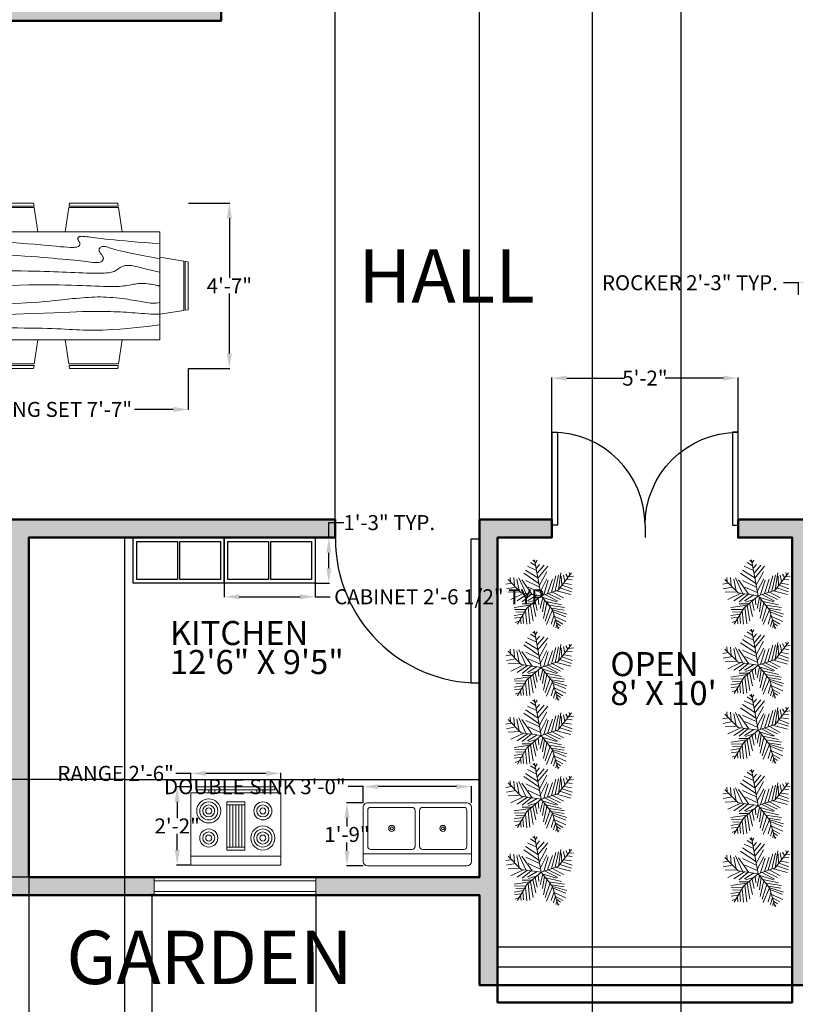
# Model space of a CAD drawing. Units: inches. Extents: x -60 to 743, y -483 to 510.
# Tile 3 of 7: x 120 to 378, y -299 to 29. Entities that reach past the tile are written whole.
import ezdxf

# ---------------------------------------------------------------- set-up
doc = ezdxf.new("R2010")
doc.units = ezdxf.units.IN
doc.header["$MEASUREMENT"] = 0
for name, color, linetype, lineweight in [('A-ANNO-DIMS', 2, 'Continuous', 18), ('A-AREA-IDEN', 7, 'Continuous', 25), ('A-DOOR', 150, 'Continuous', 25), ('A-EQPM', 40, 'Continuous', 18), ('A-FLOR-CASE', 40, 'Continuous', 25), ('A-FLOR-FIXT', 40, 'Continuous', 18), ('A-WALL-PATT', 30, 'Continuous', 13), ('FURNITURE', 40, 'Continuous', 18), ('STAIRS', 202, 'Continuous', 25), ('TREES', 80, 'Continuous', 13), ('WALL BOUNDRY', 10, 'Continuous', 50), ('WINDOW', 200, 'Continuous', 18)]:
    doc.layers.add(name, color=color, linetype=linetype, lineweight=lineweight)
doc.styles.get("Standard").update_dxf_attribs({"font": 'arial.ttf'})
doc.dimstyles.get("Standard").update_dxf_attribs({"dimtxt": 5, "dimasz": 5, "dimexe": 0.18, "dimexo": 0.0625, "dimgap": 0.09, "dimtad": 0, "dimtih": 1, "dimtoh": 1, "dimdec": 1, "dimzin": 0, "dimdsep": 46, "dimlunit": 4, "dimtxsty": 'Standard', "dimcen": 0.09, "dimadec": 0, "dimazin": 0, "dimtfac": 1, "dimtdec": 1, "dimtofl": 0, "dimtmove": 0, "dimatfit": 3, "dimfxl": 1, "dimtolj": 1, "dimtzin": 0, "dimarcsym": 0})

# ---------------------------------------------------------------- blocks, each defined once
blk = doc.blocks.new('Wall Cabinet - 18 x 36 in front')
for p, q in [((17.5, -1.5), (17.5, -16.5)), ((18.5, -16.5), (18.5, -1.5))]:
    blk.add_line(p, q)
blk.add_lwpolyline([(0, -18), (0, 0), (36, 0), (36, -18)], close=True)
for points in [[(17.5, -16.5), (1.5, -16.5), (1.5, -1.5), (17.5, -1.5)], [(18.5, -1.5), (34.5, -1.5), (34.5, -16.5), (18.5, -16.5)]]:
    blk.add_lwpolyline(points)
blk = doc.blocks.new('Range-Oven - 30 in top')
for p, q in [((0, -3), (30, -3)), ((12, -6), (18, -6)), ((13, -20), (13, -6)), ((14, -6), (14, -20)), ((15, -20), (15, -6)), ((16, -6), (16, -20)), ((17, -20), (17, -6)), ((18, -20), (12, -20)), ((6, -24), (6, -25)), ((8, -25), (8, -24)), ((22, -25), (22, -24)), ((24, -24), (24, -25))]:
    blk.add_line(p, q)
for points in [[(0, -24), (0, 0), (30, 0), (30, -24)], [(12, -21), (12, -5), (18, -5), (18, -21)], [(2, -26), (2, -25), (28, -25), (28, -26)]]:
    blk.add_lwpolyline(points, close=True)
for centre, radius in [((6, -9), 4), ((6, -9), 3), ((24, -9), 3), ((6, -9), 2), ((6, -9), 1), ((24, -9), 2), ((24, -9), 1), ((6, -18), 3), ((6, -18), 2), ((24, -18), 4), ((24, -18), 3), ((24, -18), 2), ((6, -18), 1), ((24, -18), 1)]:
    blk.add_circle(centre, radius)
blk = doc.blocks.new('Sink-double - 36 in top')
for p, q in [((-18, -4), (18, -4)), ((-0.75, -18.5), (-0.75, -6.5)), ((0.75, -6.5), (0.75, -18.5))]:
    blk.add_line(p, q)
for points in [[(-16.5, 0), (16.5, 0)], [(-18, -19.5), (-18, -1.5)], [(18, -1.5), (18, -19.5)], [(-16.5, -18.5), (-16.5, -6.5)], [(-15.5, -5.5), (-1.75, -5.5)], [(1.75, -5.5), (15.5, -5.5)], [(16.5, -6.5), (16.5, -18.5)], [(-1.75, -19.5), (-15.5, -19.5)], [(15.5, -19.5), (1.75, -19.5)], [(16.5, -21), (-16.5, -21)]]:
    blk.add_lwpolyline(points)
for centre, radius in [((-8.5, -12.5), 1), ((-8.5, -12.5), 0.5), ((8.5, -12.5), 1), ((8.5, -12.5), 0.5)]:
    blk.add_circle(centre, radius)
for centre, radius, start, end in [((-16.5, -1.5), 1.5, 90, 180), ((16.5, -1.5), 1.5, 0, 90), ((-15.5, -6.5), 1, 90, 180), ((-1.75, -6.5), 1, 0, 90), ((1.75, -6.5), 1, 90, 180), ((15.5, -6.5), 1, 0, 90), ((-16.5, -19.5), 1.5, 180, 270), ((-15.5, -18.5), 1, 180, 270), ((-1.75, -18.5), 1, 270, 0), ((1.75, -18.5), 1, 180, 270), ((15.5, -18.5), 1, 270, 0), ((16.5, -19.5), 1.5, 270, 0)]:
    blk.add_arc(centre, radius, start, end)
blk = doc.blocks.new('*U5')
for p, q in [((0, 0), (0, -100)), ((750, 0), (750, -100))]:
    blk.add_line(p, q)
blk.add_lwpolyline([(0, 0), (0, 750), (43.75, 750), (43.75, 0)], close=True)
blk.add_arc((0, 0), 750, 0, 90)
blk = doc.blocks.new('Dining Set - 36 x 72 in.')
for p, q in [((-22, 27.5), (-22.1562, 26.50042)), ((-5.8416, 26.5), (-22.1534, 26.5)), ((-22, 27.5), (-6, 27.5)), ((-5.8437, 26.49966), (-6, 27.5)), ((6, 27.5), (5.8438, 26.50042)), ((22.1584, 26.5), (5.8466, 26.5)), ((6, 27.5), (22, 27.5)), ((22.1563, 26.49966), (22, 27.5)), ((-22.2343, 26.00059), (-23.4847, 17.99762)), ((-22.2304, 26), (-5.7608, 26)), ((-4.5152, 17.99762), (-5.7655, 25.99926)), ((5.7657, 26.00059), (4.5153, 17.99762)), ((5.7696, 26), (22.2392, 26)), ((23.4848, 17.99762), (22.2345, 25.99926)), ((36, 18), (-36, 18)), ((-36, 18), (-36, -18)), ((36, -18), (36, 18)), ((-45.5, 8), (-44.5004, 8.15617)), ((-45.5, 8), (-45.5, -8)), ((-44.5, -8.15843), (-44.5, 8.15338)), ((-44.0006, 8.23428), (-35.9976, 9.48474)), ((-44, 8.23041), (-44, -8.23915)), ((44.0006, 8.23428), (35.9976, 9.48474)), ((44, 8.23041), (44, -8.23915)), ((44.5, -8.15843), (44.5, 8.15338)), ((45.5, 8), (44.5005, 8.15617)), ((45.5, 8), (45.5, -8)), ((-44.4997, -8.15631), (-45.5, -8)), ((-35.9976, -9.48476), (-43.9993, -8.2345)), ((35.9976, -9.48476), (43.9993, -8.2345)), ((44.4997, -8.15631), (45.5, -8)), ((-36, -18), (36, -18)), ((-22.2343, -26.0006), (-23.4847, -17.99762)), ((-4.5152, -17.99762), (-5.7655, -25.99928)), ((5.7657, -26.0006), (4.5153, -17.99762)), ((23.4848, -17.99762), (22.2345, -25.99928)), ((-22.2304, -26), (-5.7608, -26)), ((5.7696, -26), (22.2392, -26)), ((-22, -27.5), (-22.1562, -26.50044)), ((-5.8416, -26.5), (-22.1534, -26.5)), ((-22, -27.5), (-6, -27.5)), ((-5.8437, -26.49967), (-6, -27.5)), ((6, -27.5), (5.8438, -26.50044)), ((22.1584, -26.5), (5.8466, -26.5)), ((6, -27.5), (22, -27.5)), ((22.1563, -26.49967), (22, -27.5))]:
    blk.add_line(p, q)
for points in [[(-36, 15), (-31.1772, 14.97754), (-26.8079, 14.91406), (-22.8538, 14.81543), (-19.276, 14.6875), (-16.0362, 14.53613), (-13.0957, 14.36718), (-10.4159, 14.18652), (-7.9583, 14), (-5.6904, 13.81315), (-3.6035, 13.63021), (-1.6954, 13.45508), (0.0365, 13.29166), (1.5945, 13.14388), (2.9811, 13.01562), (4.1988, 12.9108), (5.25, 12.83333), (6.1393, 12.78613), (6.8802, 12.76823), (7.4883, 12.77767), (7.9792, 12.8125), (8.3685, 12.87077), (8.6719, 12.95052), (8.9049, 13.0498), (9.0833, 13.16666), (9.2205, 13.29899), (9.3216, 13.44401), (9.3895, 13.59879), (9.4271, 13.76041), (9.4373, 13.92594), (9.4232, 14.09245), (9.3875, 14.257), (9.3333, 14.41666), (9.2638, 14.56917), (9.1836, 14.71484), (9.0975, 14.85465), (9.0104, 14.98958), (8.9272, 15.1206), (8.8529, 15.2487), (8.7922, 15.37483), (8.75, 15.5), (8.7305, 15.62467), (8.7344, 15.74739), (8.7617, 15.86621), (8.8125, 15.97916), (8.8867, 16.08431), (8.9844, 16.17968), (9.1055, 16.26334), (9.25, 16.33333), (9.4189, 16.38802), (9.6172, 16.42708), (9.8506, 16.45052), (10.125, 16.45833), (10.4463, 16.45052), (10.8203, 16.42708), (11.2529, 16.38802), (11.75, 16.33333), (12.3184, 16.26318), (12.9694, 16.17838), (13.7151, 16.07991), (14.5677, 15.96875), (15.5395, 15.84586), (16.6426, 15.71224), (17.8893, 15.56884), (19.2917, 15.41666), (20.859, 15.25667), (22.5879, 15.08984), (24.4721, 14.91715), (26.5052, 14.73958), (28.6809, 14.5581), (30.9929, 14.3737), (33.4347, 14.18733), (36, 14)], [(-36, 10), (-28.9766, 10.14274), (-23.1725, 10.20442), (-18.4241, 10.19775), (-14.5677, 10.13541), (-11.4399, 10.03011), (-8.877, 9.89453), (-6.7154, 9.74137), (-4.7917, 9.58333), (-2.9698, 9.43082), (-1.2246, 9.28515), (0.4415, 9.14534), (2.026, 9.01041), (3.5266, 8.87939), (4.9408, 8.7513), (6.266, 8.62516), (7.5, 8.5), (8.6411, 8.37549), (9.6914, 8.2539), (10.6538, 8.13818), (11.5312, 8.03125), (12.3267, 7.93603), (13.043, 7.85547), (13.6831, 7.79248), (14.25, 7.75), (14.7471, 7.7303), (15.1797, 7.73307), (15.5537, 7.75732), (15.875, 7.80208), (16.1494, 7.86637), (16.3828, 7.94922), (16.5811, 8.04964), (16.75, 8.16666), (16.8944, 8.29915), (17.0143, 8.44531), (17.1089, 8.60319), (17.1771, 8.77083), (17.218, 8.94629), (17.2305, 9.1276), (17.2137, 9.31282), (17.1667, 9.5), (17.0895, 9.6875), (16.987, 9.875), (16.8649, 10.0625), (16.7292, 10.25), (16.5856, 10.4375), (16.4401, 10.625), (16.2985, 10.8125), (16.1667, 11), (16.05, 11.18733), (15.9518, 11.3737), (15.8752, 11.5581), (15.8229, 11.73958), (15.798, 11.91715), (15.8034, 12.08984), (15.842, 12.25667), (15.9167, 12.41666), (16.0295, 12.56836), (16.1784, 12.70833), (16.3605, 12.83268), (16.5729, 12.9375), (16.8127, 13.01888), (17.0768, 13.07291), (17.3625, 13.0957), (17.6667, 13.08333), (17.9894, 13.03312), (18.3418, 12.94726), (18.7382, 12.82918), (19.1927, 12.68229), (19.7195, 12.51001), (20.3327, 12.31575), (21.0465, 12.10294), (21.875, 11.875), (22.8357, 11.63354), (23.959, 11.37304), (25.2786, 11.08618), (26.8282, 10.76562), (28.6414, 10.40405), (30.752, 9.99414), (33.1936, 9.52856), (36, 9)], [(-36, 5.5), (-30.7157, 5.3348), (-26.069, 5.20963), (-21.9946, 5.11767), (-18.4271, 5.05208), (-15.3009, 5.00602), (-12.5508, 4.97265), (-10.1112, 4.94515), (-7.9167, 4.91666), (-5.909, 4.88167), (-4.0586, 4.83984), (-2.3429, 4.79215), (-0.7396, 4.73958), (0.7739, 4.6831), (2.22, 4.6237), (3.6213, 4.56233), (5, 4.5), (6.373, 4.43782), (7.7344, 4.3776), (9.0723, 4.32129), (10.375, 4.27083), (11.6309, 4.22819), (12.8281, 4.19531), (13.9551, 4.17415), (15, 4.16666), (15.954, 4.17448), (16.819, 4.19791), (17.6001, 4.23698), (18.3021, 4.29166), (18.9299, 4.36198), (19.4883, 4.44791), (19.9823, 4.54948), (20.4167, 4.66666), (20.7969, 4.79899), (21.1302, 4.94401), (21.4245, 5.09879), (21.6875, 5.26041), (21.9271, 5.42594), (22.1511, 5.59245), (22.3672, 5.757), (22.5834, 5.91666), (22.8065, 6.06868), (23.0404, 6.21093), (23.2879, 6.34147), (23.5521, 6.45833), (23.8358, 6.55957), (24.142, 6.64323), (24.4735, 6.70735), (24.8334, 6.75), (25.2235, 6.76969), (25.642, 6.76692), (26.0858, 6.74267), (26.5521, 6.69791), (27.0379, 6.63362), (27.5404, 6.55078), (28.0565, 6.45036), (28.5834, 6.33333), (29.1242, 6.19987), (29.7071, 6.04687), (30.3661, 5.87044), (31.1354, 5.66666), (32.0493, 5.43164), (33.142, 5.16146), (34.4475, 4.85221), (36, 4.5)], [(-36, -1), (-30.7915, -0.6591), (-26.0195, -0.38216), (-21.6519, -0.16284), (-17.6563, 0.00521), (-14.0005, 0.12833), (-10.6523, 0.21289), (-7.5796, 0.26522), (-4.75, 0.29166), (-2.134, 0.29793), (0.2878, 0.28711), (2.5317, 0.26163), (4.6146, 0.22396), (6.5529, 0.17651), (8.3633, 0.12174), (10.0623, 0.06209), (11.6667, 0), (13.1899, -0.06201), (14.6341, -0.1211), (15.9982, -0.17432), (17.2813, -0.21875), (18.4823, -0.25147), (19.6003, -0.26953), (20.6343, -0.27002), (21.5834, -0.25), (22.4481, -0.20768), (23.2357, -0.14584), (23.9549, -0.06836), (24.6146, 0.02083), (25.2235, 0.11784), (25.7904, 0.21875), (26.3241, 0.31966), (26.8334, 0.41666), (27.3265, 0.50618), (27.8099, 0.58593), (28.2894, 0.65397), (28.7709, 0.70833), (29.2601, 0.74707), (29.763, 0.76823), (30.2855, 0.76985), (30.8334, 0.75), (31.4088, 0.70784), (31.9994, 0.64713), (32.589, 0.57275), (33.1615, 0.48958), (33.7008, 0.4025), (34.1908, 0.3164), (34.6153, 0.23616), (34.9584, 0.16666), (35.2099, 0.11165), (35.3848, 0.07031), (35.504, 0.04069), (35.5886, 0.02083), (35.6594, 0.00879), (35.7377, 0.0026), (35.8442, 0.00032), (36, 0)], [(-36, -6.5), (-27.1843, -6.31267), (-20.084, -6.1263), (-14.469, -5.9419), (-10.1094, -5.76042), (-6.7752, -5.58285), (-4.2363, -5.41016), (-2.2629, -5.24333), (-0.625, -5.08334), (0.8708, -4.93099), (2.2715, -4.78646), (3.5872, -4.64974), (4.8281, -4.52084), (6.0046, -4.39974), (7.127, -4.28646), (8.2053, -4.18099), (9.25, -4.08334), (10.2705, -3.99382), (11.2734, -3.91407), (12.2647, -3.84603), (13.25, -3.79167), (14.2354, -3.75293), (15.2266, -3.73177), (16.2295, -3.73015), (17.25, -3.75), (18.2912, -3.79248), (19.3451, -3.85547), (20.4009, -3.93604), (21.4479, -4.03125), (22.4754, -4.13819), (23.4727, -4.25391), (24.4289, -4.37549), (25.3334, -4.5), (26.1785, -4.62492), (26.9694, -4.74935), (27.7145, -4.87281), (28.4219, -4.99479), (29.1, -5.11483), (29.7572, -5.23242), (30.4016, -5.34709), (31.0417, -5.45834), (31.6837, -5.56437), (32.3262, -5.65821), (32.9658, -5.73153), (33.599, -5.77604), (34.2224, -5.78345), (34.8327, -5.74545), (35.4264, -5.65373), (36, -5.5)], [(-36, -10), (-26.4022, -9.81299), (-18.4675, -9.62891), (-11.9839, -9.45069), (-6.7396, -9.28125), (-2.5226, -9.12354), (0.8789, -8.98047), (3.6769, -8.85498), (6.0833, -8.75), (8.2767, -8.66765), (10.3021, -8.60677), (12.1712, -8.56543), (13.8958, -8.54167), (15.4876, -8.53353), (16.9583, -8.53907), (18.3197, -8.55632), (19.5834, -8.58334), (20.7616, -8.61841), (21.8685, -8.66081), (22.9188, -8.71004), (23.9271, -8.76563), (24.9081, -8.82707), (25.8763, -8.89388), (26.8465, -8.96558), (27.8334, -9.04167), (28.8474, -9.12118), (29.8828, -9.20117), (30.93, -9.27824), (31.9792, -9.34896), (33.0205, -9.40991), (34.0443, -9.45768), (35.0407, -9.48885), (36, -9.5)], [(-36, -14.5), (-30.0881, -14.33513), (-25.0332, -14.21224), (-20.7312, -14.12647), (-17.0781, -14.07292), (-13.97, -14.04671), (-11.3027, -14.04297), (-8.9724, -14.05681), (-6.875, -14.08334), (-4.9224, -14.11833), (-3.0905, -14.16016), (-1.3709, -14.20785), (0.2448, -14.26042), (1.7647, -14.3169), (3.1973, -14.3763), (4.5507, -14.43767), (5.8333, -14.5), (7.0554, -14.5621), (8.235, -14.62175), (9.3922, -14.67652), (10.5469, -14.72396), (11.7192, -14.76164), (12.929, -14.78711), (14.1965, -14.79794), (15.5417, -14.79167), (16.9933, -14.76424), (18.6152, -14.70508), (20.4804, -14.60197), (22.6615, -14.44271), (25.2312, -14.21509), (28.2624, -13.9069), (31.8277, -13.50594), (36, -13)]]:
    blk.add_lwpolyline(points)
blk = doc.blocks.new('*U21')
for p, q in [((-221.9198, 1197.3052), (-433.5526, 1338.8594)), ((-258.7244, 1362.456), (-332.3336, 1421.4348)), ((0, 0), (-266.7, 1447.8)), ((-231.1146, 1315.2628), (-166.7002, 1421.4348)), ((-194.31, 1102.9442), (-65.4812, 1256.284)), ((-148.3106, 914.1968), (118.5418, 1220.9018)), ((-93.091, 489.5342), (-700.3796, 902.3858)), ((-129.8956, 713.6638), (-626.7704, 1032.1544)), ((-185.1152, 1008.5578), (-553.1612, 1185.4942)), ((-129.8956, 701.8528), (265.7602, 1185.4942)), ((-74.7014, 418.7444), (219.7608, 961.39)), ((412.9786, 147.447), (587.8068, 796.2392)), ((560.197, 182.8292), (698.2206, 819.8358)), ((685.8, 228.6), (1219.2, 914.4)), ((689.0258, 230.0224), (790.2448, 914.1968)), ((891.4384, 831.6214), (946.658, 572.1096)), ((983.4626, 867.0036), (1066.2666, 725.4494)), ((1121.4862, 925.9824), (1149.0706, 831.6214)), ((-1206.4492, 501.3198), (-1418.082, 465.9376)), ((-800.1, 114.3), (-1333.5, 647.7)), ((-1234.059, 536.7274), (-1252.4486, 737.2604)), ((-1105.2302, 725.4494), (-1077.6458, 395.1732)), ((-976.4268, 666.4706), (-884.4026, 194.6402)), ((-902.8176, 713.6638), (-617.5756, 100.2538)), ((-369.1382, 53.086), (-783.1836, 642.874)), ((-617.5756, 607.4918), (-74.7014, 347.98)), ((-28.6766, 171.0436), (228.9556, 678.2816)), ((100.1268, 41.275), (284.1498, 619.2774)), ((256.5654, 88.4682), (449.7832, 666.4706)), ((808.6344, 784.4282), (827.0494, 418.7444)), ((845.439, 418.7444), (1241.0948, 277.1902)), ((919.0482, 501.3198), (1222.6798, 454.152)), ((1029.462, 654.685), (1241.0948, 631.0884)), ((1112.2914, 760.8316), (1296.3144, 784.4282)), ((-1031.621, 347.98), (-1399.667, 277.1902)), ((-847.598, 159.2326), (-1326.0578, 135.636)), ((-718.7946, 88.4682), (-1215.644, -147.447)), ((-543.9664, 76.6572), (-967.2066, -206.4512)), ((0, 0), (-800.1, 114.3)), ((-405.9428, 53.086), (-764.794, -241.8334)), ((0, 0), (-571.5, -495.3)), ((-166.7002, 29.4894), (-543.9664, -206.4512)), ((-525.5514, 347.98), (-28.6766, 123.8504)), ((0, 0), (685.8, 228.6)), ((0, 0), (457.2, -571.5)), ((164.5412, 41.275), (661.416, -218.2368)), ((284.1498, 88.4682), (781.0246, -147.447)), ((458.978, 147.447), (891.4384, -88.4682)), ((615.4166, 194.6402), (1185.8752, 41.275)), ((753.4148, 312.5978), (1222.6798, 159.2326)), ((-442.7474, -383.3876), (-1086.8406, -477.7486)), ((-387.5278, -324.4088), (-764.794, -324.4088)), ((-166.7002, -147.447), (-507.1618, -253.619)), ((-433.5526, -383.3876), (-323.1134, -1020.3688)), ((-341.5284, -289.0012), (-221.9198, -831.6214)), ((-240.3094, -218.2368), (-157.5054, -595.7062)), ((-120.7008, -88.4682), (-93.091, -371.5766)), ((63.3222, -76.6826), (-37.8714, -513.1308)), ((44.9326, -64.897), (615.4166, -241.8334)), ((127.7366, -159.258), (54.1274, -654.685)), ((228.9556, -289.0012), (90.932, -914.1968)), ((192.151, -230.0224), (817.8292, -371.5766)), ((311.7596, -383.3876), (937.4378, -477.7486)), ((-718.7946, -737.2604), (-1086.8406, -796.2392)), ((-617.5756, -548.5384), (-1077.6458, -560.324)), ((-681.9646, -666.496), (-1022.4262, -654.685)), ((-571.5, -495.3), (-952.5, -1143)), ((-737.1842, -784.4536), (-709.5744, -1114.7298)), ((-635.9652, -607.5172), (-580.771, -1150.1374)), ((-525.5514, -465.963), (-451.9422, -1126.5408)), ((357.759, -430.5554), (164.5412, -1020.3688)), ((458.978, -572.1096), (210.5406, -1161.923)), ((514.1976, -772.6426), (403.7838, -1138.3264)), ((412.9786, -501.3452), (919.0482, -583.9206)), ((457.2, -571.5), (685.8, -1333.5)), ((468.1982, -572.1096), (1029.462, -737.2604)), ((486.5878, -642.8994), (983.4626, -843.4324)), ((-783.1836, -867.029), (-1077.6458, -902.4112)), ((-875.2078, -1008.5832), (-1040.8412, -1079.3476)), ((-829.2084, -937.7934), (-810.7934, -1126.5408)), ((578.612, -961.39), (495.7826, -1232.7128)), ((541.8074, -831.6214), (992.6574, -1032.1544)), ((578.612, -973.1756), (873.0488, -1138.3264)), ((624.6114, -1161.923), (587.8068, -1291.6916)), ((624.6114, -1102.9442), (781.0246, -1209.1162)), ((679.8056, -1268.095), (716.6102, -1291.6916))]:
    blk.add_line(p, q)
blk = doc.blocks.new('*D26')
at = {"layer": 'A-ANNO-DIMS', "color": 0, "lineweight": -2, "transparency": 16777216}
for p, q in [((188.17, -158.78), (188.17, -163.44)), ((218.45, -158.78), (218.45, -163.44)), ((193.17, -163.26), (213.45, -163.26)), ((218.45, -163.26), (223.45, -163.26))]:
    blk.add_line(p, q, dxfattribs=at)
at = {"layer": 'A-ANNO-DIMS', "color": 0, "transparency": 16777216}
for points in [[(193.17, -162.43), (193.17, -164.09), (188.17, -163.26)], [(213.45, -162.43), (213.45, -164.09), (218.45, -163.26)]]:
    blk.add_solid(points, dxfattribs=at)
at = {"layer": 'Defpoints', "color": 0, "transparency": 16777216}
for p in [(188.17, -158.72), (218.45, -158.72), (218.45, -163.26)]:
    blk.add_point(p, dxfattribs=at)
at = {"layer": 'A-ANNO-DIMS', "color": 0, "transparency": 16777216, "insert": (260.68, -163.26), "char_height": 5, "attachment_point": 5}
blk.add_mtext('\\A1;CABINET 2\'-6 1/2" TYP.', dxfattribs=at)
blk = doc.blocks.new('*D27')
at = {"layer": 'A-ANNO-DIMS', "color": 0, "lineweight": -2, "transparency": 16777216}
for p, q in [((222.99, -143.58), (222.99, -138.58)), ((222.99, -138.58), (227.99, -138.58)), ((218.51, -143.58), (223.17, -143.58)), ((222.99, -153.72), (222.99, -148.58)), ((218.51, -158.72), (223.17, -158.72))]:
    blk.add_line(p, q, dxfattribs=at)
at = {"layer": 'A-ANNO-DIMS', "color": 0, "transparency": 16777216}
for points in [[(222.16, -148.58), (223.83, -148.58), (222.99, -143.58)], [(222.16, -153.72), (223.83, -153.72), (222.99, -158.72)]]:
    blk.add_solid(points, dxfattribs=at)
at = {"layer": 'Defpoints', "color": 0, "transparency": 16777216}
for p in [(218.45, -143.58), (222.99, -143.58), (218.45, -158.72)]:
    blk.add_point(p, dxfattribs=at)
at = {"layer": 'A-ANNO-DIMS', "color": 0, "transparency": 16777216, "insert": (243.09, -138.58), "char_height": 5, "attachment_point": 5}
blk.add_mtext('\\A1;1\'-3" TYP.', dxfattribs=at)
blk = doc.blocks.new('*D34')
at = {"layer": 'A-ANNO-DIMS', "color": 0, "lineweight": -2, "transparency": 16777216}
for p, q in [((379.23, -58.74), (374.23, -58.74)), ((379.23, -62.73), (379.23, -58.56)), ((401.23, -58.74), (384.23, -58.74)), ((406.23, -62.73), (406.23, -58.56))]:
    blk.add_line(p, q, dxfattribs=at)
at = {"layer": 'A-ANNO-DIMS', "color": 0, "transparency": 16777216}
for points in [[(384.23, -57.91), (384.23, -59.58), (379.23, -58.74)], [(401.23, -57.91), (401.23, -59.58), (406.23, -58.74)]]:
    blk.add_solid(points, dxfattribs=at)
at = {"layer": 'Defpoints', "color": 0, "transparency": 16777216}
for p in [(379.23, -58.74), (379.23, -62.79), (406.23, -62.79)]:
    blk.add_point(p, dxfattribs=at)
at = {"layer": 'A-ANNO-DIMS', "color": 0, "transparency": 16777216, "insert": (343.12, -58.74), "char_height": 5, "attachment_point": 5}
blk.add_mtext('\\A1;ROCKER 2\'-3" TYP.', dxfattribs=at)
blk = doc.blocks.new('*D58')
at = {"layer": 'A-ANNO-DIMS', "color": 0, "lineweight": -2, "transparency": 16777216}
for p, q in [((177.04, -222.05), (172.04, -222.05)), ((177.04, -226.49), (177.04, -221.87)), ((202.04, -222.05), (182.04, -222.05)), ((207.04, -226.49), (207.04, -221.87))]:
    blk.add_line(p, q, dxfattribs=at)
at = {"layer": 'A-ANNO-DIMS', "color": 0, "transparency": 16777216}
for points in [[(182.04, -221.22), (182.04, -222.88), (177.04, -222.05)], [(202.04, -221.22), (202.04, -222.88), (207.04, -222.05)]]:
    blk.add_solid(points, dxfattribs=at)
at = {"layer": 'Defpoints', "color": 0, "transparency": 16777216}
for p in [(177.04, -222.05), (177.04, -226.55), (207.04, -226.55)]:
    blk.add_point(p, dxfattribs=at)
at = {"layer": 'A-ANNO-DIMS', "color": 0, "transparency": 16777216, "insert": (152.05, -222.05), "char_height": 5, "attachment_point": 5}
blk.add_mtext('\\A1;RANGE 2\'-6"', dxfattribs=at)
blk = doc.blocks.new('*D59')
at = {"layer": 'A-ANNO-DIMS', "color": 0, "lineweight": -2, "transparency": 16777216}
for p, q in [((176.98, -226.55), (172.36, -226.55)), ((172.54, -231.55), (172.54, -236.95)), ((172.54, -247.55), (172.54, -242.15)), ((176.98, -252.55), (172.36, -252.55))]:
    blk.add_line(p, q, dxfattribs=at)
at = {"layer": 'A-ANNO-DIMS', "color": 0, "transparency": 16777216}
for points in [[(171.71, -231.55), (173.38, -231.55), (172.54, -226.55)], [(171.71, -247.55), (173.38, -247.55), (172.54, -252.55)]]:
    blk.add_solid(points, dxfattribs=at)
at = {"layer": 'Defpoints', "color": 0, "transparency": 16777216}
for p in [(177.04, -226.55), (172.54, -252.55), (177.04, -252.55)]:
    blk.add_point(p, dxfattribs=at)
at = {"layer": 'A-ANNO-DIMS', "color": 0, "transparency": 16777216, "insert": (172.54, -239.55), "char_height": 5, "attachment_point": 5}
blk.add_mtext('\\A1;2\'-2"', dxfattribs=at)
blk = doc.blocks.new('*D60')
at = {"layer": 'A-ANNO-DIMS', "color": 0, "lineweight": -2, "transparency": 16777216}
for p, q in [((234.43, -226.46), (229.43, -226.46)), ((234.43, -231.8), (234.43, -226.28)), ((265.43, -226.46), (239.43, -226.46)), ((270.43, -231.8), (270.43, -226.28))]:
    blk.add_line(p, q, dxfattribs=at)
at = {"layer": 'A-ANNO-DIMS', "color": 0, "transparency": 16777216}
for points in [[(239.43, -225.63), (239.43, -227.29), (234.43, -226.46)], [(265.43, -225.63), (265.43, -227.29), (270.43, -226.46)]]:
    blk.add_solid(points, dxfattribs=at)
at = {"layer": 'Defpoints', "color": 0, "transparency": 16777216}
for p in [(234.43, -226.46), (234.43, -231.86), (270.43, -231.86)]:
    blk.add_point(p, dxfattribs=at)
at = {"layer": 'A-ANNO-DIMS', "color": 0, "transparency": 16777216, "insert": (198.37, -226.46), "char_height": 5, "attachment_point": 5}
blk.add_mtext('\\A1;DOUBLE SINK 3\'-0"', dxfattribs=at)
blk = doc.blocks.new('*D61')
at = {"layer": 'A-ANNO-DIMS', "color": 0, "lineweight": -2, "transparency": 16777216}
for p, q in [((234.37, -231.86), (228.85, -231.86)), ((229.03, -236.86), (229.03, -239.72)), ((229.03, -247.86), (229.03, -245)), ((234.37, -252.86), (228.85, -252.86))]:
    blk.add_line(p, q, dxfattribs=at)
at = {"layer": 'A-ANNO-DIMS', "color": 0, "transparency": 16777216}
for points in [[(228.2, -236.86), (229.87, -236.86), (229.03, -231.86)], [(228.2, -247.86), (229.87, -247.86), (229.03, -252.86)]]:
    blk.add_solid(points, dxfattribs=at)
at = {"layer": 'Defpoints', "color": 0, "transparency": 16777216}
for p in [(234.43, -231.86), (229.03, -252.86), (234.43, -252.86)]:
    blk.add_point(p, dxfattribs=at)
at = {"layer": 'A-ANNO-DIMS', "color": 0, "transparency": 16777216, "insert": (229.03, -242.36), "char_height": 5, "attachment_point": 5}
blk.add_mtext('\\A1;1\'-9"', dxfattribs=at)
blk = doc.blocks.new('*D62')
at = {"layer": 'A-ANNO-DIMS', "color": 0, "lineweight": -2, "transparency": 16777216}
for p, q in [((85.25, -87.32), (85.25, -101.08)), ((176.25, -87.32), (176.25, -101.08)), ((90.25, -100.9), (103.18, -100.9)), ((171.25, -100.9), (158.32, -100.9))]:
    blk.add_line(p, q, dxfattribs=at)
at = {"layer": 'A-ANNO-DIMS', "color": 0, "transparency": 16777216}
for points in [[(90.25, -100.07), (90.25, -101.74), (85.25, -100.9)], [(171.25, -100.07), (171.25, -101.74), (176.25, -100.9)]]:
    blk.add_solid(points, dxfattribs=at)
at = {"layer": 'Defpoints', "color": 0, "transparency": 16777216}
for p in [(85.25, -87.25), (176.25, -87.25), (176.25, -100.9)]:
    blk.add_point(p, dxfattribs=at)
at = {"layer": 'A-ANNO-DIMS', "color": 0, "transparency": 16777216, "insert": (130.75, -100.9), "char_height": 5, "attachment_point": 5}
blk.add_mtext('\\A1;DINING SET 7\'-7"', dxfattribs=at)
blk = doc.blocks.new('*D63')
at = {"layer": 'A-ANNO-DIMS', "color": 0, "lineweight": -2, "transparency": 16777216}
for p, q in [((176.31, -32.25), (190.08, -32.25)), ((189.9, -37.25), (189.9, -57.16)), ((189.9, -82.25), (189.9, -62.34)), ((176.31, -87.25), (190.08, -87.25))]:
    blk.add_line(p, q, dxfattribs=at)
at = {"layer": 'A-ANNO-DIMS', "color": 0, "transparency": 16777216}
for points in [[(189.07, -37.25), (190.73, -37.25), (189.9, -32.25)], [(189.07, -82.25), (190.73, -82.25), (189.9, -87.25)]]:
    blk.add_solid(points, dxfattribs=at)
at = {"layer": 'Defpoints', "color": 0, "transparency": 16777216}
for p in [(176.25, -32.25), (189.9, -32.25), (176.25, -87.25)]:
    blk.add_point(p, dxfattribs=at)
at = {"layer": 'A-ANNO-DIMS', "color": 0, "transparency": 16777216, "insert": (189.9, -59.75), "char_height": 5, "attachment_point": 5}
blk.add_mtext('\\A1;4\'-7"', dxfattribs=at)
blk = doc.blocks.new('*D69')
at = {"layer": 'A-ANNO-DIMS', "color": 0, "lineweight": -2, "transparency": 16777216}
for p, q in [((310.62, 340.16), (310.62, -473.51)), ((340.15, 340.16), (340.15, -473.51)), ((305.62, -473.33), (300.62, -473.33)), ((345.15, -473.33), (350.15, -473.33))]:
    blk.add_line(p, q, dxfattribs=at)
at = {"layer": 'A-ANNO-DIMS', "color": 0, "transparency": 16777216}
for points in [[(305.62, -472.5), (305.62, -474.17), (310.62, -473.33)], [(345.15, -472.5), (345.15, -474.17), (340.15, -473.33)]]:
    blk.add_solid(points, dxfattribs=at)
at = {"layer": 'Defpoints', "color": 0, "transparency": 16777216}
for p in [(310.62, 340.23), (340.15, 340.23), (340.15, -473.33)]:
    blk.add_point(p, dxfattribs=at)
at = {"layer": 'A-ANNO-DIMS', "color": 0, "transparency": 16777216, "insert": (325.38, -473.33), "char_height": 5, "attachment_point": 5}
blk.add_mtext('\\A1;2\'-5 1/2"', dxfattribs=at)
blk = doc.blocks.new('*D76')
at = {"layer": 'A-ANNO-DIMS', "color": 0, "lineweight": -2, "transparency": 16777216}
for p, q in [((154.99, -224.11), (154.99, -473.51)), ((123.15, -256.64), (123.15, -473.51)), ((128.15, -473.33), (132.29, -473.33)), ((149.99, -473.33), (145.85, -473.33))]:
    blk.add_line(p, q, dxfattribs=at)
at = {"layer": 'A-ANNO-DIMS', "color": 0, "transparency": 16777216}
for points in [[(128.15, -472.5), (128.15, -474.17), (123.15, -473.33)], [(149.99, -472.5), (149.99, -474.17), (154.99, -473.33)]]:
    blk.add_solid(points, dxfattribs=at)
at = {"layer": 'Defpoints', "color": 0, "transparency": 16777216}
for p in [(154.99, -224.05), (123.15, -256.58), (154.99, -473.33)]:
    blk.add_point(p, dxfattribs=at)
at = {"layer": 'A-ANNO-DIMS', "color": 0, "transparency": 16777216, "insert": (139.07, -473.33), "char_height": 5, "attachment_point": 5}
blk.add_mtext('\\A1;2\'-8"', dxfattribs=at)
blk = doc.blocks.new('*D77')
at = {"layer": 'A-ANNO-DIMS', "color": 0, "lineweight": -2, "transparency": 16777216}
for p, q in [((154.93, -224.05), (-36.93, -224.05)), ((-36.75, -229.05), (-36.75, -237.64)), ((-36.75, -251.58), (-36.75, -242.99)), ((123.08, -256.58), (-36.93, -256.58))]:
    blk.add_line(p, q, dxfattribs=at)
at = {"layer": 'A-ANNO-DIMS', "color": 0, "transparency": 16777216}
for points in [[(-37.58, -229.05), (-35.91, -229.05), (-36.75, -224.05)], [(-37.58, -251.58), (-35.91, -251.58), (-36.75, -256.58)]]:
    blk.add_solid(points, dxfattribs=at)
at = {"layer": 'Defpoints', "color": 0, "transparency": 16777216}
for p in [(154.99, -224.05), (-36.75, -256.58), (123.15, -256.58)]:
    blk.add_point(p, dxfattribs=at)
at = {"layer": 'A-ANNO-DIMS', "color": 0, "transparency": 16777216, "insert": (-36.75, -240.31), "char_height": 5, "attachment_point": 5}
blk.add_mtext('\\A1;2\'-8 1/2"', dxfattribs=at)
blk = doc.blocks.new('*D78')
at = {"layer": 'A-ANNO-DIMS', "color": 0, "lineweight": -2, "transparency": 16777216}
for p, q in [((225.15, -143.52), (225.15, 465.7)), ((230.15, 465.52), (242.31, 465.52)), ((268.15, 465.52), (255.98, 465.52)), ((273.15, -143.91), (273.15, 465.7))]:
    blk.add_line(p, q, dxfattribs=at)
at = {"layer": 'A-ANNO-DIMS', "color": 0, "transparency": 16777216}
for points in [[(230.15, 466.36), (230.15, 464.69), (225.15, 465.52)], [(268.15, 466.36), (268.15, 464.69), (273.15, 465.52)]]:
    blk.add_solid(points, dxfattribs=at)
at = {"layer": 'Defpoints', "color": 0, "transparency": 16777216}
for p in [(273.15, 465.52), (225.15, -143.58), (273.15, -143.98)]:
    blk.add_point(p, dxfattribs=at)
at = {"layer": 'A-ANNO-DIMS', "color": 0, "transparency": 16777216, "insert": (249.15, 465.52), "char_height": 5, "attachment_point": 5}
blk.add_mtext('\\A1;4\'-0"', dxfattribs=at)
blk = doc.blocks.new('*D79')
at = {"layer": 'A-ANNO-DIMS', "color": 0, "lineweight": -2, "transparency": 16777216}
for p, q in [((164.13, -262.18), (164.13, -473.51)), ((218.7, -262.64), (218.7, -473.51)), ((169.13, -473.33), (178.75, -473.33)), ((213.7, -473.33), (204.07, -473.33))]:
    blk.add_line(p, q, dxfattribs=at)
at = {"layer": 'A-ANNO-DIMS', "color": 0, "transparency": 16777216}
for points in [[(169.13, -472.5), (169.13, -474.17), (164.13, -473.33)], [(213.7, -472.5), (213.7, -474.17), (218.7, -473.33)]]:
    blk.add_solid(points, dxfattribs=at)
at = {"layer": 'Defpoints', "color": 0, "transparency": 16777216}
for p in [(164.13, -262.12), (218.7, -262.58), (218.7, -473.33)]:
    blk.add_point(p, dxfattribs=at)
at = {"layer": 'A-ANNO-DIMS', "color": 0, "transparency": 16777216, "insert": (191.41, -473.33), "char_height": 5, "attachment_point": 5}
blk.add_mtext('\\A1;4\'-6 1/2"', dxfattribs=at)
blk = doc.blocks.new('*D82')
at = {"layer": 'A-ANNO-DIMS', "color": 0, "lineweight": -2, "transparency": 16777216}
for p, q in [((297.15, -137.52), (297.15, -90.3)), ((302.15, -90.48), (321.41, -90.48)), ((354.15, -90.48), (334.88, -90.48)), ((359.15, -137.52), (359.15, -90.3))]:
    blk.add_line(p, q, dxfattribs=at)
at = {"layer": 'A-ANNO-DIMS', "color": 0, "transparency": 16777216}
for points in [[(302.15, -89.64), (302.15, -91.31), (297.15, -90.48)], [(354.15, -89.64), (354.15, -91.31), (359.15, -90.48)]]:
    blk.add_solid(points, dxfattribs=at)
at = {"layer": 'Defpoints', "color": 0, "transparency": 16777216}
for p in [(359.15, -90.48), (297.15, -137.58), (359.15, -137.58)]:
    blk.add_point(p, dxfattribs=at)
at = {"layer": 'A-ANNO-DIMS', "color": 0, "transparency": 16777216, "insert": (328.15, -90.48), "char_height": 5, "attachment_point": 5}
blk.add_mtext('\\A1;5\'-2"', dxfattribs=at)

msp = doc.modelspace()

# ---------------------------------------------------------------- hatches: boundary and pattern name
at = {"layer": 'A-WALL-PATT'}
h = msp.add_hatch(color=256, dxfattribs=at)
h.dxf.hatch_style = 1
h.paths.add_polyline_path([(412.35, 168.77), (415.89, 168.77), (415.89, 114.92), (412.35, 114.92)], flags=16)
h.paths.add_polyline_path([(87.81, -138.81), (87.81, -142.35), (48.31, -142.32), (48.31, -138.78)], flags=16)
h.paths.add_polyline_path([(459.53, -138.78), (513.39, -138.78), (513.39, -142.32), (459.53, -142.32)], flags=16)
h.paths.add_polyline_path([(164.84, -257.78), (218.7, -257.78), (218.7, -261.32), (164.84, -261.32)], flags=16)
h.paths.add_polyline_path([(417.15, 114.92), (415.89, 114.92), (415.89, 168.77), (417.15, 168.77), (417.15, 195.42), (411.15, 195.42), (411.15, 168.77), (412.35, 168.77), (412.35, 114.92), (411.15, 114.92), (411.15, 28.42), (610.15, 28.42), (610.15, -43.58), (508.15, -43.58), (508.15, -49.58), (610.15, -49.58), (610.15, -137.58), (513.39, -137.58), (513.39, -138.78), (459.53, -138.78), (459.53, -137.58), (359.15, -137.58), (359.15, -143.58), (377.15, -143.58), (377.15, -292.58), (383.15, -292.58), (383.15, -143.58), (459.53, -143.58), (459.53, -142.32), (513.39, -142.32), (513.39, -143.58), (610.15, -143.58), (610.15, -415.58), (610.15, -421.58), (616.15, -421.58), (616.15, 418.42), (13.15, 418.42), (13.15, -421.58), (19.15, -421.58), (430.15, -421.58), (430.15, -415.58), (19.15, -415.58), (19.15, -143.58), (48.31, -143.58), (48.31, -142.32), (87.81, -142.35), (87.81, -143.58), (117.15, -143.58), (117.15, -262.58), (164.84, -262.58), (164.84, -261.32), (218.7, -261.32), (218.7, -262.58), (273.15, -262.58), (273.15, -292.58), (279.15, -292.58), (279.15, -143.58), (297.15, -143.58), (297.15, -137.58), (273.15, -137.58), (273.15, -256.58), (218.7, -256.58), (218.7, -257.78), (164.84, -257.78), (164.84, -256.58), (123.15, -256.58), (123.15, -143.58), (225.15, -143.58), (225.15, -137.58), (87.81, -137.58), (87.81, -138.81), (48.31, -138.78), (48.31, -137.58), (19.15, -137.58), (19.15, 28.42), (187.15, 28.42), (187.15, 34.42), (19.15, 34.42), (19.15, 178.42), (273.15, 178.42), (273.15, 184.42), (19.15, 184.42), (19.15, 345.58), (195.14, 345.58), (195.14, 348.9), (19.15, 348.9), (19.15, 412.42), (267.15, 412.42), (267.15, 319.83), (273.15, 319.83), (273.15, 412.42), (411.15, 412.42), (411.15, 376.24), (417.15, 376.24), (417.15, 412.42), (610.15, 412.42), (610.15, 249.42), (411.15, 249.42), (411.15, 243.42), (610.15, 243.42), (610.15, 34.42), (417.15, 34.42)])
h = msp.add_hatch(color=256, dxfattribs=at)
h.dxf.hatch_style = 1
h.paths.add_polyline_path([(273.15, 265.98), (267.15, 265.98), (267.15, 232.42), (273.15, 232.42)])
h.paths.add_polyline_path([(417.15, 322.39), (411.15, 322.39), (411.15, 297.42), (417.15, 297.42)])
h.paths.add_polyline_path([(417.15, 195.42), (411.15, 195.42), (411.15, 168.77), (417.15, 168.77)])
h.paths.add_polyline_path([(459.53, -137.58), (359.15, -137.58), (359.15, -143.58), (377.15, -143.58), (377.15, -292.58), (383.15, -292.58), (383.15, -143.58), (459.53, -143.58)])
h.paths.add_polyline_path([(279.15, -143.58), (297.15, -143.58), (297.15, -137.58), (273.15, -137.58), (273.15, -256.58), (218.7, -256.58), (218.7, -262.58), (273.15, -262.58), (273.15, -292.58), (279.15, -292.58)])
h.paths.add_polyline_path([(123.15, -143.58), (225.15, -143.58), (225.15, -137.58), (87.81, -137.58), (87.81, -143.58), (117.15, -143.58), (117.15, -262.58), (164.84, -262.58), (164.84, -256.58), (123.15, -256.58)])
h = msp.add_hatch(color=256, dxfattribs=at)
h.dxf.hatch_style = 1
h.paths.add_polyline_path([(48.31, -138.78), (87.81, -138.81), (87.81, -142.35), (48.31, -142.32)], flags=17)
h.paths.add_polyline_path([(164.84, -257.78), (218.7, -257.78), (218.7, -261.32), (164.84, -261.32)], flags=17)
h.paths.add_polyline_path([(48.31, -142.32), (87.81, -142.35), (87.81, -138.81), (48.31, -138.78)])
h.paths.add_polyline_path([(164.84, -261.32), (218.7, -261.32), (218.7, -257.78), (164.84, -257.78)])

# ---------------------------------------------------------------- linework, layer by layer
at = {"layer": 'A-FLOR-CASE'}
msp.add_lwpolyline([(154.99, -143.58), (154.99, -224.05), (273.15, -224.05)], dxfattribs=at)
at = {"layer": 'STAIRS'}
for p, q in [((279.15, -279.79), (377.15, -279.79)), ((279.15, -286.41), (377.15, -286.41))]:
    msp.add_line(p, q, dxfattribs=at)
at = {"layer": 'WALL BOUNDRY'}
msp.add_lwpolyline([(610.15, -415.58), (610.15, -421.58), (616.15, -421.58), (616.15, 418.42), (13.15, 418.42), (13.15, -421.58), (19.15, -421.58), (430.15, -421.58), (430.15, -415.58), (19.15, -415.58), (19.15, -143.58), (117.15, -143.58), (117.15, -262.58), (273.15, -262.58), (273.15, -292.58), (279.15, -292.58), (377.15, -292.58), (383.15, -292.58), (383.15, -143.58), (610.15, -143.58)], close=True, dxfattribs=at)
msp.add_lwpolyline([(610.15, -137.58), (359.15, -137.58), (359.15, -143.58), (377.15, -143.58), (377.15, -298.27), (279.15, -298.27), (279.15, -143.58), (297.15, -143.58), (297.15, -137.58), (273.15, -137.58), (273.15, -256.58), (123.15, -256.58), (123.15, -143.58), (225.15, -143.58), (225.15, -137.58), (19.15, -137.58), (19.15, 28.42), (187.15, 28.42), (187.15, 34.42)], dxfattribs=at)
at = {"layer": 'WINDOW'}
for points in [[(218.7, -256.58), (218.7, -262.58), (164.84, -262.58), (164.84, -256.58)], [(218.7, -257.78), (218.7, -261.32), (164.84, -261.32), (164.84, -257.78)]]:
    msp.add_lwpolyline(points, close=True, dxfattribs=at)

# ---------------------------------------------------------------- block references
at = {"layer": 'A-DOOR', "yscale": 0.0412653609199711, "zscale": 0.0412653609199711}
for p, xscale in [((297.25, -139.45), 0.0412653609199711), ((359.15, -139.45), -0.0412653609199711)]:
    msp.add_blockref('*U5', p, dxfattribs=dict(at, xscale=xscale))
at = {"layer": 'A-DOOR', "xscale": 0.063986642508199, "yscale": 0.063986642508199, "zscale": 0.063986642508199, "rotation": 180}
msp.add_blockref('*U5', (273.15, -143.98), dxfattribs=at)
at = {"layer": 'A-EQPM', "rotation": 180}
msp.add_blockref('Range-Oven - 30 in top', (207.04, -252.55), dxfattribs=at)
at = {"layer": 'A-FLOR-CASE', "xscale": 0.8411327527354037, "yscale": 0.8411327527354037, "zscale": 0.8411327527354037}
for p in [(157.89, -143.58), (188.17, -143.58)]:
    msp.add_blockref('Wall Cabinet - 18 x 36 in front', p, dxfattribs=at)
at = {"layer": 'A-FLOR-FIXT', "rotation": 180}
msp.add_blockref('Sink-double - 36 in top', (252.43, -252.86), dxfattribs=at)
at = {"layer": 'FURNITURE'}
msp.add_blockref('Dining Set - 36 x 72 in.', (130.75, -59.75), dxfattribs=at)
at = {"layer": 'TREES', "xscale": 0.0082811290650079, "yscale": 0.0082811290650079, "zscale": 0.0082811290650079}
for p in [(293.65, -162.9), (365.79, -162.9), (293.65, -186.75), (365.79, -186.01), (365.79, -207.7), (293.65, -209.47), (293.65, -230.6), (365.79, -232.75), (293.65, -254.93), (365.79, -255.42)]:
    msp.add_blockref('*U21', p, dxfattribs=at)

# ---------------------------------------------------------------- texts
at = {"layer": 'A-AREA-IDEN'}
for s, height, p in [('HALL', 17.752, (232.83, -65.34)), ('KITCHEN ', 8, (170.13, -179.33)), ('12\'6" X 9\'5"', 8, (170.13, -188.97)), ('OPEN', 8, (316.66, -189.67)), ("8' X 10'", 8, (316.66, -199.31)), ('GARDEN', 17.752, (135.65, -292.17))]:
    msp.add_text(s, height=height, dxfattribs=at).set_placement(p)

# ---------------------------------------------------------------- dimensions: what is measured, and where the dimension line sits
at = {"layer": 'A-ANNO-DIMS'}
for base, p1, p2, picture, middle in [((273.15, 465.52), (225.15, -143.58), (273.15, -143.98), '*D78', (249.15, 465.52)), ((340.15, -473.33), (310.62, 340.23), (340.15, 340.23), '*D69', (325.38, -473.33)), ((359.15, -90.48), (297.15, -137.58), (359.15, -137.58), '*D82', (328.15, -90.48)), ((154.99, -473.33), (123.15, -256.58), (154.99, -224.05), '*D76', (139.07, -473.33)), ((218.7, -473.33), (164.13, -262.12), (218.7, -262.58), '*D79', (191.41, -473.33))]:
    dim = msp.add_linear_dim(base=base, p1=p1, p2=p2, dimstyle='Standard', override={"dimdec": 1, "dimlfac": 1, "dimrnd": 0, "dimzin": 1, "dimdsep": 46, "dimlunit": 4, "dimfrac": 2}, dxfattribs=at)
    dim.commit()
    dim.dimension.update_dxf_attribs({"geometry": picture, "text_midpoint": middle})
for base, p1, p2, angle, picture, middle in [((189.9, -32.25), (176.25, -87.25), (176.25, -32.25), 90, '*D63', (189.9, -59.75)), ((-36.75, -256.58), (154.99, -224.05), (123.15, -256.58), 90, '*D77', (-36.75, -240.31)), ((172.54, -252.55), (177.04, -226.55), (177.04, -252.55), 270, '*D59', (172.54, -239.55)), ((229.03, -252.86), (234.43, -231.86), (234.43, -252.86), 270, '*D61', (229.03, -242.36))]:
    dim = msp.add_linear_dim(base=base, p1=p1, p2=p2, angle=angle, dimstyle='Standard', override={"dimdec": 1, "dimlfac": 1, "dimrnd": 0, "dimzin": 1, "dimdsep": 46, "dimlunit": 4, "dimfrac": 2}, dxfattribs=at)
    dim.commit()
    dim.dimension.update_dxf_attribs({"geometry": picture, "text_midpoint": middle})
for base, p1, p2, angle, text, picture, middle in [((379.23, -58.74), (406.23, -62.79), (379.23, -62.79), 180, 'ROCKER <> TYP.', '*D34', (343.12, -58.74)), ((222.99, -143.58), (218.45, -158.72), (218.45, -143.58), 90, '<> TYP.', '*D27', (243.09, -138.58)), ((177.04, -222.05), (207.04, -226.55), (177.04, -226.55), 180, 'RANGE <>', '*D58', (152.05, -222.05)), ((234.43, -226.46), (270.43, -231.86), (234.43, -231.86), 180, 'DOUBLE SINK <>', '*D60', (198.37, -226.46))]:
    dim = msp.add_linear_dim(base=base, p1=p1, p2=p2, angle=angle, text=text, dimstyle='Standard', override={"dimdec": 1, "dimlfac": 1, "dimrnd": 0, "dimzin": 1, "dimdsep": 46, "dimlunit": 4, "dimfrac": 2}, dxfattribs=at)
    dim.commit()
    dim.dimension.update_dxf_attribs({"geometry": picture, "text_midpoint": middle})
for base, p1, p2, text, picture, middle in [((176.25, -100.9), (85.25, -87.25), (176.25, -87.25), 'DINING SET <>', '*D62', (130.75, -100.9)), ((218.45, -163.26), (188.17, -158.72), (218.45, -158.72), 'CABINET <> TYP.', '*D26', (260.68, -163.26))]:
    dim = msp.add_linear_dim(base=base, p1=p1, p2=p2, text=text, dimstyle='Standard', override={"dimdec": 1, "dimlfac": 1, "dimrnd": 0, "dimzin": 1, "dimdsep": 46, "dimlunit": 4, "dimfrac": 2}, dxfattribs=at)
    dim.commit()
    dim.dimension.update_dxf_attribs({"geometry": picture, "text_midpoint": middle})

doc.saveas('drawing.dxf')
